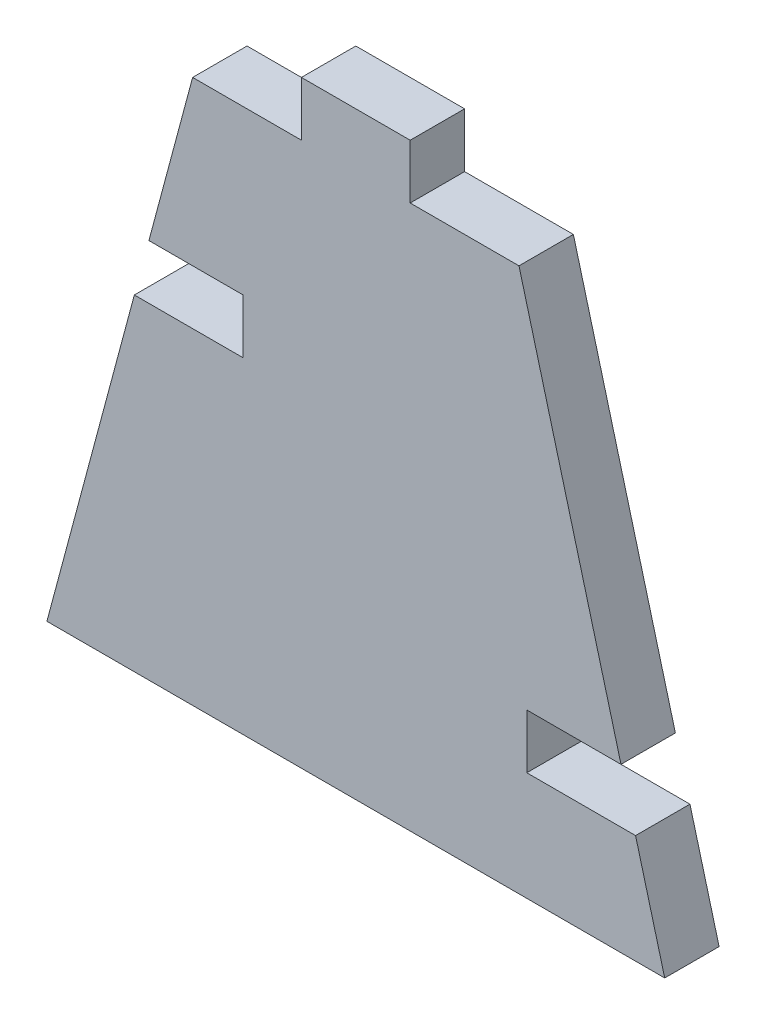
SolidWorks part; units mm, degrees
material "Plain Carbon Steel"
ref_plane "Front Plane" through (0, 0, 0) normal (0, 0, 1) x (1, 0, 0)
ref_plane "Top Plane" through (0, 0, 0) normal (0, 1, 0) x (1, 0, 0)
ref_plane "Right Plane" through (0, 0, 0) normal (1, 0, 0) x (0, 0, -1)
sketch "Leg Profile Sketch" plane through (0, 0, 0) normal (0, 0, 1) x (1, 0, 0)
  line L0 (0, 0) -> (113.5898, 0)
  line L15 (56.7949, 0) -> (56.7949, 117.2542) construction
  line L16 (0, 0) -> (16.077, 60)
  line L17 (26.7949, 100) -> (46.7949, 100)
  line L18 (46.7949, 100) -> (46.7949, 110)
  line L19 (46.7949, 110) -> (66.7949, 110)
  line L20 (66.7949, 100) -> (66.7949, 110)
  line L21 (86.7949, 100) -> (66.7949, 100)
  line L22 (113.5898, 0) -> (108.2309, 20)
  line L23 (16.077, 60) -> (36.077, 60)
  line L24 (36.077, 60) -> (36.077, 70)
  line L25 (36.077, 70) -> (18.7564, 70)
  line L26 (108.2309, 20) -> (88.2309, 20)
  line L27 (88.2309, 20) -> (88.2309, 30)
  line L28 (88.2309, 30) -> (105.5514, 30)
  line L29 (18.7564, 70) -> (26.7949, 100)
  line L30 (105.5514, 30) -> (86.7949, 100)
  point P10 (56.7949, 110)
  dimension "D1" = 30
  dimension "D2" = 10
  dimension "D3" = 100
  dimension "D4" = 75
  dimension "D5" = 60
  dimension "D6" = 20
  dimension "D7" = 10
  dimension "D8" = 20
  dimension "D9" = 20
  dimension "D10" = 10
  dimension "D11" = 110
extrude "Leg Plate 10mm" add sketch "Leg Profile Sketch" along normal mid plane 10
